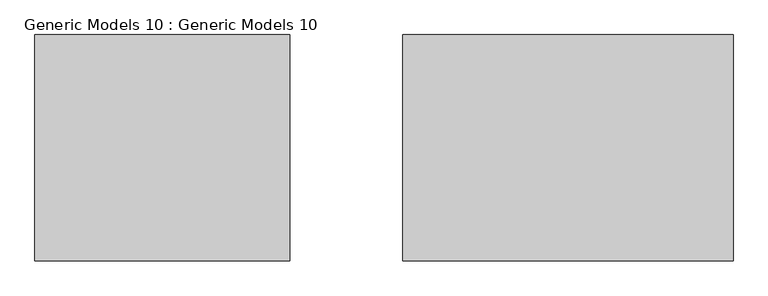
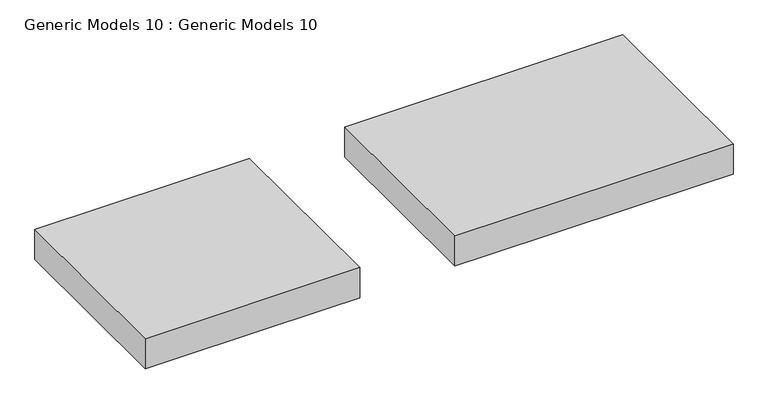
"""IFC4 building model written with IfcOpenShell, lengths in millimetres: proxy geometry, Generic Models 10 : Generic Models 10."""

from ifc_helpers import new_model, si_unit, frame, origin, place, context, project, spatial, polyline, outline, extrude, source, transform, mapped, element, save


def generic_models_10_generic_models_10_998b1f2c(model_context):
    return source(origin(), model_context, "Body", "SweptSolid", [
        extrude(outline(polyline([(5238.75, -38282.6645004), (5238.75, -38130.2645004), (5238.75, -37406.3645004), (5238.75, -37253.9645004), (5391.15, -37253.9645004), (5391.15, -38282.6645004), (5238.75, -38282.6645004)])), frame((0.0, 19682.7756148, 0.0), z_axis=(0.0, 1.0, 0.0), x_axis=(0.0, 0.0, 1.0)), (0.0, 0.0, 1.0), 914.4),
        extrude(outline(polyline([(5238.75, -35463.2645004), (5391.15, -35463.2645004), (5391.15, -36796.7645004), (5238.75, -36796.7645004), (5238.75, -36644.3645004), (5238.75, -35615.6645004), (5238.75, -35463.2645004)])), frame((0.0, 19682.7756148, 0.0), z_axis=(0.0, 1.0, 0.0), x_axis=(0.0, 0.0, 1.0)), (0.0, 0.0, 1.0), 914.4),
    ])


if __name__ == "__main__":
    model = new_model("IFC4")
    model_context = context("Model", 3, world=origin())
    ifc_project = project(units=[si_unit("LENGTHUNIT", "METRE", prefix="MILLI")], contexts=[model_context])
    site = spatial("IfcSite", under=ifc_project)
    building = spatial("IfcBuilding", under=site)
    placement = place(None, origin())
    generic_models_10_generic_models_10_shape = generic_models_10_generic_models_10_998b1f2c(model_context)
    element("IfcBuildingElementProxy", 1, Name="Generic Models 10 : Generic Models 10", ObjectType="Generic Models 10 : Generic Models 10", at=placement, inside=building, context=model_context, shape_type="MappedRepresentation", body=[
        mapped(generic_models_10_generic_models_10_shape, transform((0.0, 0.0, 0.0), x_axis=(1.0, 0.0, 0.0), y_axis=(0.0, 1.0, 0.0), z_axis=(0.0, 0.0, 1.0))),
    ])
    save(model, "model.ifc")
